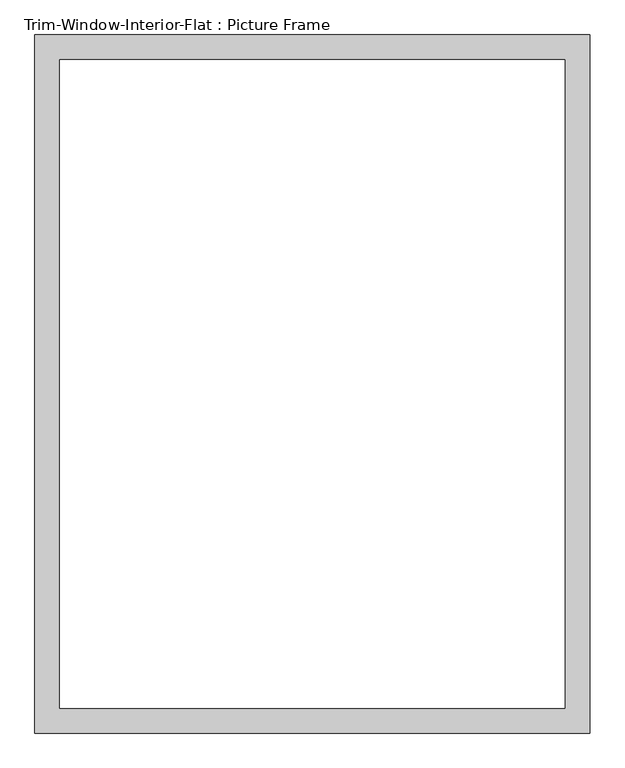
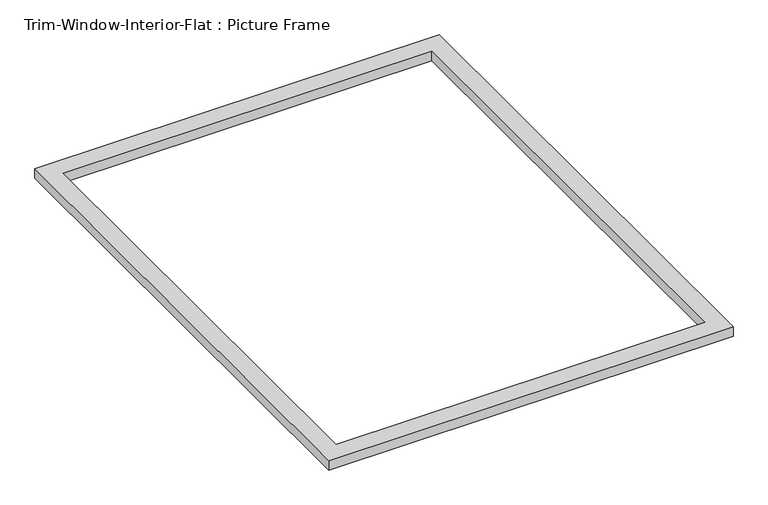
"""IFC4 building model written with IfcOpenShell, lengths in millimetres: proxy geometry, Trim-Window-Interior-Flat : Picture Frame."""

from ifc_helpers import new_model, si_unit, origin, origin_with_axes, place, context, project, spatial, polyline, outline, extrude, source, transform, mapped, element, save


def trim_window_interior_flat_picture_frame_d5efd988(model_context):
    return source(origin(), model_context, "Body", "SweptSolid", [
        extrude(outline(polyline([(641.35, 44.45), (641.35, -1568.45), (-641.35, -1568.45), (-641.35, 44.45), (641.35, 44.45)]), holes=[polyline([(584.2, -12.7), (-584.2, -12.7), (-584.2, -1511.3), (584.2, -1511.3), (584.2, -12.7)])]), origin_with_axes(), (0.0, 0.0, 1.0), 31.75),
    ])


if __name__ == "__main__":
    model = new_model("IFC4")
    model_context = context("Model", 3, world=origin())
    ifc_project = project(units=[si_unit("LENGTHUNIT", "METRE", prefix="MILLI")], contexts=[model_context])
    site = spatial("IfcSite", under=ifc_project)
    building = spatial("IfcBuilding", under=site)
    placement = place(None, origin())
    trim_window_interior_flat_picture_frame_shape = trim_window_interior_flat_picture_frame_d5efd988(model_context)
    element("IfcBuildingElementProxy", 1, Name="Trim-Window-Interior-Flat : Picture Frame", ObjectType="Trim-Window-Interior-Flat : Picture Frame", at=placement, inside=building, context=model_context, shape_type="MappedRepresentation", body=[
        mapped(trim_window_interior_flat_picture_frame_shape, transform((0.0, 0.0, 0.0), x_axis=(1.0, 0.0, 0.0), y_axis=(0.0, 1.0, 0.0), z_axis=(0.0, 0.0, 1.0))),
    ])
    save(model, "model.ifc")

# Revit data of these elements
# Type "Trim-Window-Interior-Flat : Picture Frame"
#   Trim Thickness_Picture Frame = 0' - 1 1/4"
#   Trim Width = 0' - 2 1/4"
#   Trim Thickness_with Sill = 0' - 0 3/4"
#   Sill Thickness = 0' - 1 1/4"
#   Opening Width [instance default] = 2' - 0"
#   Opening Height [instance default] = 3' - 0"
#   Default Elevation = 4' - 0"
#   Sill = no
#   Picture Frame = yes
#   Trim Material [instance default] = none
# Element 1 (IfcBuildingElementProxy, "Trim-Window-Interior-Flat : Picture Frame")
#   Opening Width = 3' - 11"
#   Opening Height = 5' - 0"
#   Trim Material = Wood - Stained
#   Materials on its faces: "Wood - Stained"
# Materials
#   "Wood - Stained": class "Wood", colour RGB 224 178 126, transparency 0, Cost = 0
